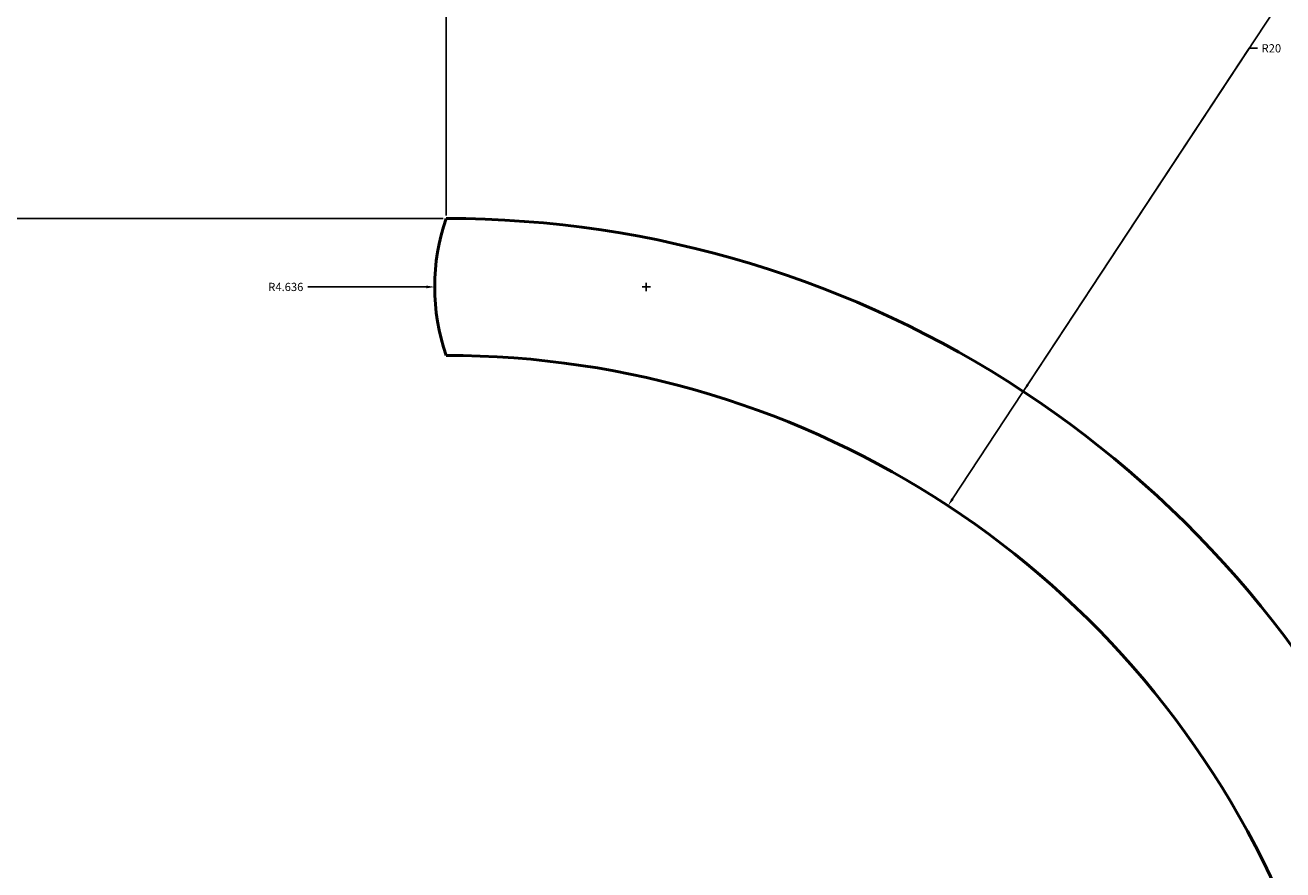
# Model space of a CAD drawing. Units: inches. Extents: x -14 to 108, y -9 to 83.
# Tile 10 of 13: x 38 to 65, y 46 to 64. Entities that reach past the tile are written whole.
import ezdxf

# ---------------------------------------------------------------- set-up
doc = ezdxf.new("R2010")
doc.units = ezdxf.units.IN
doc.header["$MEASUREMENT"] = 0
doc.layers.add('M-DIMS', color=2, linetype='Continuous', lineweight=18)
doc.layers.add('M-OUTL', color=7, linetype='Continuous', lineweight=50)
doc.styles.get("Standard").update_dxf_attribs({"font": 'arial.ttf'})
doc.dimstyles.get("Standard").update_dxf_attribs({"dimtxt": 0.18, "dimasz": 0.18, "dimexe": 0.18, "dimexo": 0.0625, "dimgap": 0.09, "dimtad": 0, "dimtih": 1, "dimtoh": 1, "dimzin": 0, "dimdsep": 46, "dimtxsty": 'Standard', "dimcen": 0.09, "dimadec": 0, "dimazin": 0, "dimtfac": 1, "dimtofl": 0, "dimtmove": 0, "dimatfit": 3, "dimfxl": 1, "dimtolj": 1, "dimtzin": 0, "dimarcsym": 0})

# ---------------------------------------------------------------- blocks, each defined once
blk = doc.blocks.new('*D12')
at = {"layer": 'Defpoints', "color": 0, "transparency": 16777216}
for p in [(86.478, 57.664), (107.813, 57.664), (47.098, 37.119)]:
    blk.add_point(p, dxfattribs=at)
at = {"layer": 'M-DIMS', "color": 0, "lineweight": -2, "transparency": 16777216}
for p, q in [((86.541, 57.664), (107.993, 57.664)), ((107.813, 57.484), (107.813, 47.573)), ((107.813, 37.299), (107.813, 47.21)), ((47.16, 37.119), (107.993, 37.119))]:
    blk.add_line(p, q, dxfattribs=at)
at = {"layer": 'M-DIMS', "color": 0, "transparency": 16777216}
for points in [[(107.783, 57.484), (107.843, 57.484), (107.813, 57.664)], [(107.783, 37.299), (107.843, 37.299), (107.813, 37.119)]]:
    blk.add_solid(points, dxfattribs=at)
at = {"layer": 'M-DIMS', "color": 0, "transparency": 16777216, "insert": (107.813, 47.392), "char_height": 0.18, "attachment_point": 5}
blk.add_mtext('\\A1;20.544', dxfattribs=at)
blk = doc.blocks.new('*D15')
at = {"layer": 'Defpoints', "color": 0, "transparency": 16777216}
for p in [(47.098, 82.834), (47.098, 60.119), (26.462, 55.756)]:
    blk.add_point(p, dxfattribs=at)
at = {"layer": 'M-DIMS', "color": 0, "lineweight": -2, "transparency": 16777216}
for p, q in [((26.462, 55.818), (26.462, 83.014)), ((47.098, 60.182), (47.098, 83.014)), ((26.642, 82.834), (36.315, 82.834)), ((46.918, 82.834), (37.245, 82.834))]:
    blk.add_line(p, q, dxfattribs=at)
at = {"layer": 'M-DIMS', "color": 0, "transparency": 16777216}
for points in [[(26.642, 82.864), (26.642, 82.804), (26.462, 82.834)], [(46.918, 82.864), (46.918, 82.804), (47.098, 82.834)]]:
    blk.add_solid(points, dxfattribs=at)
at = {"layer": 'M-DIMS', "color": 0, "transparency": 16777216, "insert": (36.78, 82.834), "char_height": 0.18, "attachment_point": 5}
blk.add_mtext('\\A1;20.636', dxfattribs=at)
blk = doc.blocks.new('*D22')
at = {"layer": 'Defpoints', "color": 0, "transparency": 16777216}
for p in [(67.492, 82.834), (47.098, 60.119), (67.492, 47.754)]:
    blk.add_point(p, dxfattribs=at)
at = {"layer": 'M-DIMS', "color": 0, "lineweight": -2, "transparency": 16777216}
for p, q in [((47.098, 60.182), (47.098, 83.014)), ((67.492, 47.817), (67.492, 83.014)), ((47.278, 82.834), (56.83, 82.834)), ((67.312, 82.834), (57.76, 82.834))]:
    blk.add_line(p, q, dxfattribs=at)
at = {"layer": 'M-DIMS', "color": 0, "transparency": 16777216}
for points in [[(47.278, 82.864), (47.278, 82.804), (47.098, 82.834)], [(67.312, 82.864), (67.312, 82.804), (67.492, 82.834)]]:
    blk.add_solid(points, dxfattribs=at)
at = {"layer": 'M-DIMS', "color": 0, "transparency": 16777216, "insert": (57.295, 82.834), "char_height": 0.18, "attachment_point": 5}
blk.add_mtext('\\A1;20.394', dxfattribs=at)
blk = doc.blocks.new('*D23')
at = {"layer": 'Defpoints', "color": 0, "transparency": 16777216}
for p in [(-13.617, 60.119), (47.098, 60.119), (26.462, 55.756)]:
    blk.add_point(p, dxfattribs=at)
at = {"layer": 'M-DIMS', "color": 0, "lineweight": -2, "transparency": 16777216}
for p, q in [((47.035, 60.119), (-13.797, 60.119)), ((-13.617, 59.939), (-13.617, 58.119)), ((-13.617, 55.936), (-13.617, 57.756)), ((26.399, 55.756), (-13.797, 55.756))]:
    blk.add_line(p, q, dxfattribs=at)
at = {"layer": 'M-DIMS', "color": 0, "transparency": 16777216}
for points in [[(-13.647, 59.939), (-13.587, 59.939), (-13.617, 60.119)], [(-13.647, 55.936), (-13.587, 55.936), (-13.617, 55.756)]]:
    blk.add_solid(points, dxfattribs=at)
at = {"layer": 'M-DIMS', "color": 0, "transparency": 16777216, "insert": (-13.617, 57.937), "char_height": 0.18, "attachment_point": 5}
blk.add_mtext('\\A1;4.364', dxfattribs=at)
blk = doc.blocks.new('*D30')
at = {"layer": 'Defpoints', "color": 0, "transparency": 16777216}
for p in [(59.745, 56.33), (47.098, 37.119)]:
    blk.add_point(p, dxfattribs=at)
at = {"layer": 'M-DIMS', "color": 0, "lineweight": -2, "transparency": 16777216}
for p, q in [((67.333, 67.856), (59.844, 56.48)), ((67.513, 67.856), (67.333, 67.856)), ((47.098, 37.029), (47.098, 37.209)), ((47.008, 37.119), (47.188, 37.119))]:
    blk.add_line(p, q, dxfattribs=at)
at = {"layer": 'M-DIMS', "color": 0, "transparency": 16777216}
blk.add_solid([(59.819, 56.497), (59.869, 56.464), (59.745, 56.33)], dxfattribs=at)
at = {"layer": 'M-DIMS', "color": 0, "transparency": 16777216, "insert": (67.818, 67.856), "char_height": 0.18, "attachment_point": 5}
blk.add_mtext('\\A1;R23', dxfattribs=at)
blk = doc.blocks.new('*D31')
at = {"layer": 'Defpoints', "color": 0, "transparency": 16777216}
for p in [(58.096, 53.824), (47.098, 37.119)]:
    blk.add_point(p, dxfattribs=at)
at = {"layer": 'M-DIMS', "color": 0, "lineweight": -2, "transparency": 16777216}
for p, q in [((64.695, 63.847), (58.195, 53.974)), ((64.875, 63.847), (64.695, 63.847)), ((47.098, 37.029), (47.098, 37.209)), ((47.008, 37.119), (47.188, 37.119))]:
    blk.add_line(p, q, dxfattribs=at)
at = {"layer": 'M-DIMS', "color": 0, "transparency": 16777216}
blk.add_solid([(58.17, 53.991), (58.22, 53.958), (58.096, 53.824)], dxfattribs=at)
at = {"layer": 'M-DIMS', "color": 0, "transparency": 16777216, "insert": (65.18, 63.847), "char_height": 0.18, "attachment_point": 5}
blk.add_mtext('\\A1;R20', dxfattribs=at)
blk = doc.blocks.new('*D32')
at = {"layer": 'Defpoints', "color": 0, "transparency": 16777216}
for p in [(46.849, 58.619), (51.484, 58.619)]:
    blk.add_point(p, dxfattribs=at)
at = {"layer": 'M-DIMS', "color": 0, "lineweight": -2, "transparency": 16777216}
for p, q in [((51.484, 58.529), (51.484, 58.709)), ((44.067, 58.619), (46.669, 58.619)), ((51.394, 58.619), (51.574, 58.619))]:
    blk.add_line(p, q, dxfattribs=at)
at = {"layer": 'M-DIMS', "color": 0, "transparency": 16777216}
blk.add_solid([(46.669, 58.649), (46.669, 58.589), (46.849, 58.619)], dxfattribs=at)
at = {"layer": 'M-DIMS', "color": 0, "transparency": 16777216, "insert": (43.587, 58.619), "char_height": 0.18, "attachment_point": 5}
blk.add_mtext('\\A1;R4.636', dxfattribs=at)

msp = doc.modelspace()

# ---------------------------------------------------------------- linework, layer by layer
at = {"layer": 'M-OUTL'}
for centre, radius, start, end in [((51.4841, 58.6193), 4.6356, 161.12031, 198.87969), ((47.0979, 37.1193), 23, 23.2807, 90), ((47.0979, 37.1193), 20, 23.2807, 90)]:
    msp.add_arc(centre, radius, start, end, dxfattribs=at)

# ---------------------------------------------------------------- dimensions: what is measured, and where the dimension line sits
at = {"layer": 'M-DIMS'}
for base, p1, p2, picture, middle in [((47.0979, 82.8343), (26.4616, 55.7556), (47.0979, 60.1193), '*D15', (36.7798, 82.8343)), ((67.4915, 82.8343), (47.0979, 60.1193), (67.4915, 47.7542), '*D22', (57.2947, 82.8343))]:
    dim = msp.add_linear_dim(base=base, p1=p1, p2=p2, dimstyle='Standard', override={"dimdec": 3, "dimlfac": 1, "dimrnd": 0, "dimzin": 0, "dimdsep": 46, "dimlunit": 2}, dxfattribs=at)
    dim.commit()
    dim.dimension.update_dxf_attribs({"geometry": picture, "text_midpoint": middle})
for center, mpoint, override, picture, middle in [((47.0979, 37.1193), (59.745, 56.33), {"dimdec": 0, "dimlfac": 1, "dimrnd": 0, "dimzin": 0, "dimdsep": 46, "dimlunit": 2}, '*D30', (67.8183, 67.8564)), ((47.0979, 37.1193), (58.0959, 53.8239), {"dimdec": 0, "dimlfac": 1, "dimrnd": 0, "dimzin": 0, "dimdsep": 46, "dimlunit": 2}, '*D31', (65.1795, 63.8467)), ((51.4841, 58.6193), (46.8485, 58.619), {"dimdec": 3, "dimlfac": 1, "dimrnd": 0, "dimzin": 0, "dimdsep": 46, "dimlunit": 2}, '*D32', (44.0672, 58.6188))]:
    dim = msp.add_radius_dim(center=center, mpoint=mpoint, dimstyle='Standard', override=override, dxfattribs=at)
    dim.commit()
    dim.dimension.update_dxf_attribs({"geometry": picture, "text_midpoint": middle, "dimtype": 164})
for base, p1, p2, picture, middle in [((-13.6171, 60.1193), (26.4616, 55.7556), (47.0979, 60.1193), '*D23', (-13.6171, 57.9375)), ((107.8129, 57.6637), (47.0979, 37.1193), (86.4784, 57.6637), '*D12', (107.8129, 47.3915))]:
    dim = msp.add_linear_dim(base=base, p1=p1, p2=p2, angle=90, dimstyle='Standard', override={"dimdec": 3, "dimlfac": 1, "dimrnd": 0, "dimzin": 0, "dimdsep": 46, "dimlunit": 2}, dxfattribs=at)
    dim.commit()
    dim.dimension.update_dxf_attribs({"geometry": picture, "text_midpoint": middle})

doc.saveas('drawing.dxf')
